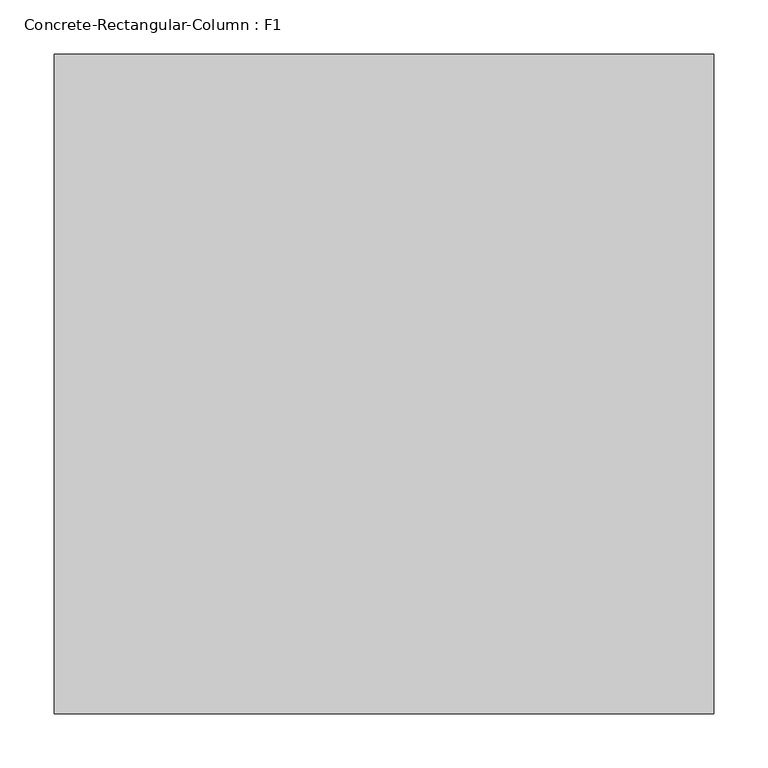
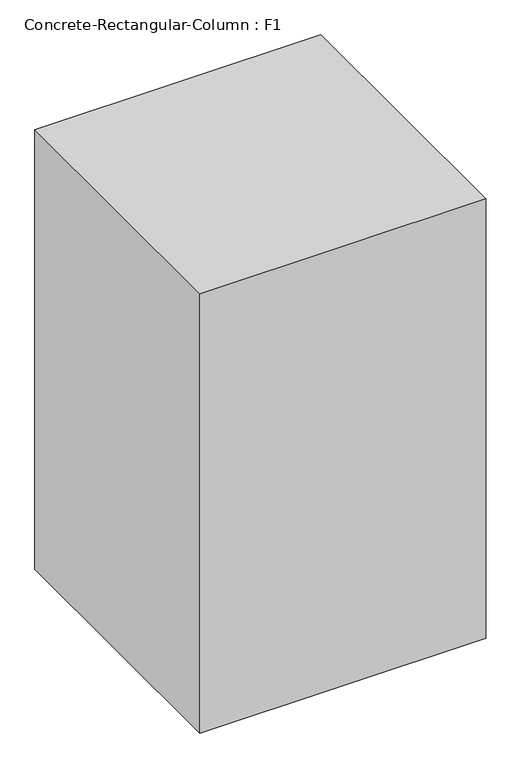
"""IFC4 building model written with IfcOpenShell, lengths in millimetres: column geometry, Concrete-Rectangular-Column : F1."""

from ifc_helpers import new_model, si_unit, origin, origin_with_axes, place, context, project, spatial, polyline, outline, extrude, source, transform, mapped, element, save


def concrete_rectangular_column_f1_2b960ed8(model_context):
    return source(origin(), model_context, "Body", "SweptSolid", [
        extrude(outline(polyline([(304.8, 304.8), (304.8, -304.8), (-304.8, -304.8), (-304.8, 304.8), (304.8, 304.8)])), origin_with_axes(), (0.0, 0.0, 1.0), 990.6),
    ])


if __name__ == "__main__":
    model = new_model("IFC4")
    model_context = context("Model", 3, world=origin())
    ifc_project = project(units=[si_unit("LENGTHUNIT", "METRE", prefix="MILLI")], contexts=[model_context])
    site = spatial("IfcSite", under=ifc_project)
    building = spatial("IfcBuilding", under=site)
    placement = place(None, origin())
    concrete_rectangular_column_f1_shape = concrete_rectangular_column_f1_2b960ed8(model_context)
    element("IfcColumn", 1, ObjectType="Concrete-Rectangular-Column : F1", at=placement, inside=building, context=model_context, shape_type="MappedRepresentation", body=[
        mapped(concrete_rectangular_column_f1_shape, transform((0.0, 0.0, 0.0), x_axis=(1.0, 0.0, 0.0), y_axis=(0.0, 1.0, 0.0), z_axis=(0.0, 0.0, 1.0))),
    ])
    save(model, "model.ifc")

# Revit data of these elements
# Type "Concrete-Rectangular-Column : F1"
#   b = 609.6 mm
#   h = 609.6 mm
#   Structural Material [instance default] = Concrete, Cast-in-Place gray
# Element 1 (IfcColumn, "Concrete-Rectangular-Column : F1")
#   Materials on its faces: "Concrete, Cast-in-Place gray"
# Materials
#   "Concrete, Cast-in-Place gray": class "Concrete", colour RGB 192 192 192, transparency 0, Description = "Cast-in-place concrete", Cost = 0
